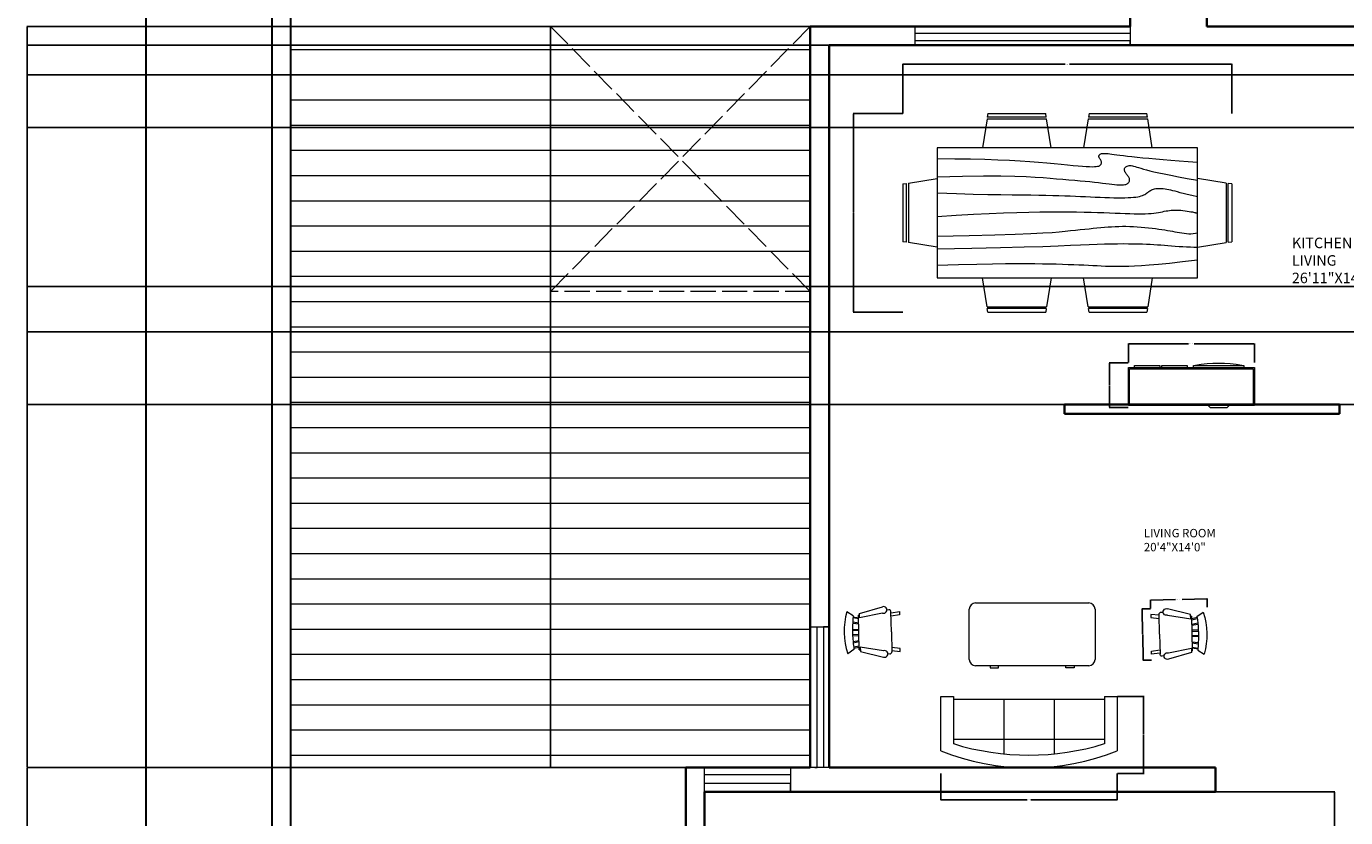
# Model space of a CAD drawing. Units: inches. Extents: x 727 to 1967, y -579 to 606.
# Tile 2 of 5: x 727 to 1355, y -78 to 299. Entities that reach past the tile are written whole.
import ezdxf

# ---------------------------------------------------------------- set-up
doc = ezdxf.new("R2010")
doc.units = ezdxf.units.IN
doc.header["$MEASUREMENT"] = 0
doc.linetypes.add('ACAD_ISO02W100', pattern=[15, 12, -3])
for name, color, linetype, lineweight in [('A-ANNO-DIMS', 2, 'Continuous', 18), ('A-AREA-IDEN', 7, 'Continuous', 18), ('A-FLOR-EXT', 7, 'Continuous', 25), ('A-FLOR-EXT-OVHD', 8, 'ACAD_ISO02W100', 18), ('A-FLOR-PATT', 9, 'Continuous', 13), ('A-FURN', 8, 'Continuous', 18), ('A-GLAZ', 4, 'Continuous', 18), ('A-WALL', 7, 'Continuous', 35), ('C-PROP', 7, 'Continuous', 30)]:
    doc.layers.add(name, color=color, linetype=linetype, lineweight=lineweight)
doc.styles.get("Standard").update_dxf_attribs({"font": 'arial.ttf'})
doc.dimstyles.get("Standard").update_dxf_attribs({"dimtxt": 0.18, "dimasz": 0.18, "dimexe": 0.18, "dimexo": 0.0625, "dimgap": 0.09, "dimtad": 0, "dimtih": 1, "dimtoh": 1, "dimdec": 4, "dimzin": 0, "dimdsep": 46, "dimtxsty": 'Standard', "dimcen": 0.09, "dimadec": 0, "dimazin": 0, "dimtfac": 1, "dimtdec": 4, "dimtofl": 0, "dimtmove": 0, "dimatfit": 3, "dimfxl": 1, "dimtolj": 1, "dimtzin": 0, "dimarcsym": 0})

# ---------------------------------------------------------------- blocks, each defined once
blk = doc.blocks.new('Dining Set - 36 x 72 in.')
for p, q in [((-22.2343, 26.00059), (-23.4847, 17.99762)), ((-22.2304, 26), (-5.7608, 26)), ((-22, 27.5), (-22.1562, 26.50042)), ((-5.8416, 26.5), (-22.1534, 26.5)), ((-22, 27.5), (-6, 27.5)), ((-5.8437, 26.49966), (-6, 27.5)), ((-4.5152, 17.99762), (-5.7655, 25.99926)), ((5.7657, 26.00059), (4.5153, 17.99762)), ((5.7696, 26), (22.2392, 26)), ((6, 27.5), (5.8438, 26.50042)), ((22.1584, 26.5), (5.8466, 26.5)), ((6, 27.5), (22, 27.5)), ((22.1563, 26.49966), (22, 27.5)), ((23.4848, 17.99762), (22.2345, 25.99926)), ((36, 18), (-36, 18)), ((-36, 18), (-36, -18)), ((36, -18), (36, 18)), ((-45.5, 8), (-44.5004, 8.15617)), ((-45.5, 8), (-45.5, -8)), ((-44.5, -8.15843), (-44.5, 8.15338)), ((-44.0006, 8.23428), (-35.9976, 9.48474)), ((-44, 8.23041), (-44, -8.23915)), ((44.0006, 8.23428), (35.9976, 9.48474)), ((44, 8.23041), (44, -8.23915)), ((44.5, -8.15843), (44.5, 8.15338)), ((45.5, 8), (44.5005, 8.15617)), ((45.5, 8), (45.5, -8)), ((-44.4997, -8.15631), (-45.5, -8)), ((-35.9976, -9.48476), (-43.9993, -8.2345)), ((35.9976, -9.48476), (43.9993, -8.2345)), ((44.4997, -8.15631), (45.5, -8)), ((-36, -18), (36, -18)), ((-22.2343, -26.0006), (-23.4847, -17.99762)), ((-4.5152, -17.99762), (-5.7655, -25.99928)), ((5.7657, -26.0006), (4.5153, -17.99762)), ((23.4848, -17.99762), (22.2345, -25.99928)), ((-22.2304, -26), (-5.7608, -26)), ((-22, -27.5), (-22.1562, -26.50044)), ((-5.8416, -26.5), (-22.1534, -26.5)), ((-22, -27.5), (-6, -27.5)), ((-5.8437, -26.49967), (-6, -27.5)), ((5.7696, -26), (22.2392, -26)), ((6, -27.5), (5.8438, -26.50044)), ((22.1584, -26.5), (5.8466, -26.5)), ((6, -27.5), (22, -27.5)), ((22.1563, -26.49967), (22, -27.5))]:
    blk.add_line(p, q)
for points in [[(-36, 15), (-31.1772, 14.97754), (-26.8079, 14.91406), (-22.8538, 14.81543), (-19.276, 14.6875), (-16.0362, 14.53613), (-13.0957, 14.36718), (-10.4159, 14.18652), (-7.9583, 14), (-5.6904, 13.81315), (-3.6035, 13.63021), (-1.6954, 13.45508), (0.0365, 13.29166), (1.5945, 13.14388), (2.9811, 13.01562), (4.1988, 12.9108), (5.25, 12.83333), (6.1393, 12.78613), (6.8802, 12.76823), (7.4883, 12.77767), (7.9792, 12.8125), (8.3685, 12.87077), (8.6719, 12.95052), (8.9049, 13.0498), (9.0833, 13.16666), (9.2205, 13.29899), (9.3216, 13.44401), (9.3895, 13.59879), (9.4271, 13.76041), (9.4373, 13.92594), (9.4232, 14.09245), (9.3875, 14.257), (9.3333, 14.41666), (9.2638, 14.56917), (9.1836, 14.71484), (9.0975, 14.85465), (9.0104, 14.98958), (8.9272, 15.1206), (8.8529, 15.2487), (8.7922, 15.37483), (8.75, 15.5), (8.7305, 15.62467), (8.7344, 15.74739), (8.7617, 15.86621), (8.8125, 15.97916), (8.8867, 16.08431), (8.9844, 16.17968), (9.1055, 16.26334), (9.25, 16.33333), (9.4189, 16.38802), (9.6172, 16.42708), (9.8506, 16.45052), (10.125, 16.45833), (10.4463, 16.45052), (10.8203, 16.42708), (11.2529, 16.38802), (11.75, 16.33333), (12.3184, 16.26318), (12.9694, 16.17838), (13.7151, 16.07991), (14.5677, 15.96875), (15.5395, 15.84586), (16.6426, 15.71224), (17.8893, 15.56884), (19.2917, 15.41666), (20.859, 15.25667), (22.5879, 15.08984), (24.4721, 14.91715), (26.5052, 14.73958), (28.6809, 14.5581), (30.9929, 14.3737), (33.4347, 14.18733), (36, 14)], [(-36, 10), (-28.9766, 10.14274), (-23.1725, 10.20442), (-18.4241, 10.19775), (-14.5677, 10.13541), (-11.4399, 10.03011), (-8.877, 9.89453), (-6.7154, 9.74137), (-4.7917, 9.58333), (-2.9698, 9.43082), (-1.2246, 9.28515), (0.4415, 9.14534), (2.026, 9.01041), (3.5266, 8.87939), (4.9408, 8.7513), (6.266, 8.62516), (7.5, 8.5), (8.6411, 8.37549), (9.6914, 8.2539), (10.6538, 8.13818), (11.5312, 8.03125), (12.3267, 7.93603), (13.043, 7.85547), (13.6831, 7.79248), (14.25, 7.75), (14.7471, 7.7303), (15.1797, 7.73307), (15.5537, 7.75732), (15.875, 7.80208), (16.1494, 7.86637), (16.3828, 7.94922), (16.5811, 8.04964), (16.75, 8.16666), (16.8944, 8.29915), (17.0143, 8.44531), (17.1089, 8.60319), (17.1771, 8.77083), (17.218, 8.94629), (17.2305, 9.1276), (17.2137, 9.31282), (17.1667, 9.5), (17.0895, 9.6875), (16.987, 9.875), (16.8649, 10.0625), (16.7292, 10.25), (16.5856, 10.4375), (16.4401, 10.625), (16.2985, 10.8125), (16.1667, 11), (16.05, 11.18733), (15.9518, 11.3737), (15.8752, 11.5581), (15.8229, 11.73958), (15.798, 11.91715), (15.8034, 12.08984), (15.842, 12.25667), (15.9167, 12.41666), (16.0295, 12.56836), (16.1784, 12.70833), (16.3605, 12.83268), (16.5729, 12.9375), (16.8127, 13.01888), (17.0768, 13.07291), (17.3625, 13.0957), (17.6667, 13.08333), (17.9894, 13.03312), (18.3418, 12.94726), (18.7382, 12.82918), (19.1927, 12.68229), (19.7195, 12.51001), (20.3327, 12.31575), (21.0465, 12.10294), (21.875, 11.875), (22.8357, 11.63354), (23.959, 11.37304), (25.2786, 11.08618), (26.8282, 10.76562), (28.6414, 10.40405), (30.752, 9.99414), (33.1936, 9.52856), (36, 9)], [(-36, 5.5), (-30.7157, 5.3348), (-26.069, 5.20963), (-21.9946, 5.11767), (-18.4271, 5.05208), (-15.3009, 5.00602), (-12.5508, 4.97265), (-10.1112, 4.94515), (-7.9167, 4.91666), (-5.909, 4.88167), (-4.0586, 4.83984), (-2.3429, 4.79215), (-0.7396, 4.73958), (0.7739, 4.6831), (2.22, 4.6237), (3.6213, 4.56233), (5, 4.5), (6.373, 4.43782), (7.7344, 4.3776), (9.0723, 4.32129), (10.375, 4.27083), (11.6309, 4.22819), (12.8281, 4.19531), (13.9551, 4.17415), (15, 4.16666), (15.954, 4.17448), (16.819, 4.19791), (17.6001, 4.23698), (18.3021, 4.29166), (18.9299, 4.36198), (19.4883, 4.44791), (19.9823, 4.54948), (20.4167, 4.66666), (20.7969, 4.79899), (21.1302, 4.94401), (21.4245, 5.09879), (21.6875, 5.26041), (21.9271, 5.42594), (22.1511, 5.59245), (22.3672, 5.757), (22.5834, 5.91666), (22.8065, 6.06868), (23.0404, 6.21093), (23.2879, 6.34147), (23.5521, 6.45833), (23.8358, 6.55957), (24.142, 6.64323), (24.4735, 6.70735), (24.8334, 6.75), (25.2235, 6.76969), (25.642, 6.76692), (26.0858, 6.74267), (26.5521, 6.69791), (27.0379, 6.63362), (27.5404, 6.55078), (28.0565, 6.45036), (28.5834, 6.33333), (29.1242, 6.19987), (29.7071, 6.04687), (30.3661, 5.87044), (31.1354, 5.66666), (32.0493, 5.43164), (33.142, 5.16146), (34.4475, 4.85221), (36, 4.5)], [(-36, -1), (-30.7915, -0.6591), (-26.0195, -0.38216), (-21.6519, -0.16284), (-17.6563, 0.00521), (-14.0005, 0.12833), (-10.6523, 0.21289), (-7.5796, 0.26522), (-4.75, 0.29166), (-2.134, 0.29793), (0.2878, 0.28711), (2.5317, 0.26163), (4.6146, 0.22396), (6.5529, 0.17651), (8.3633, 0.12174), (10.0623, 0.06209), (11.6667, 0), (13.1899, -0.06201), (14.6341, -0.1211), (15.9982, -0.17432), (17.2813, -0.21875), (18.4823, -0.25147), (19.6003, -0.26953), (20.6343, -0.27002), (21.5834, -0.25), (22.4481, -0.20768), (23.2357, -0.14584), (23.9549, -0.06836), (24.6146, 0.02083), (25.2235, 0.11784), (25.7904, 0.21875), (26.3241, 0.31966), (26.8334, 0.41666), (27.3265, 0.50618), (27.8099, 0.58593), (28.2894, 0.65397), (28.7709, 0.70833), (29.2601, 0.74707), (29.763, 0.76823), (30.2855, 0.76985), (30.8334, 0.75), (31.4088, 0.70784), (31.9994, 0.64713), (32.589, 0.57275), (33.1615, 0.48958), (33.7008, 0.4025), (34.1908, 0.3164), (34.6153, 0.23616), (34.9584, 0.16666), (35.2099, 0.11165), (35.3848, 0.07031), (35.504, 0.04069), (35.5886, 0.02083), (35.6594, 0.00879), (35.7377, 0.0026), (35.8442, 0.00032), (36, 0)], [(-36, -6.5), (-27.1843, -6.31267), (-20.084, -6.1263), (-14.469, -5.9419), (-10.1094, -5.76042), (-6.7752, -5.58285), (-4.2363, -5.41016), (-2.2629, -5.24333), (-0.625, -5.08334), (0.8708, -4.93099), (2.2715, -4.78646), (3.5872, -4.64974), (4.8281, -4.52084), (6.0046, -4.39974), (7.127, -4.28646), (8.2053, -4.18099), (9.25, -4.08334), (10.2705, -3.99382), (11.2734, -3.91407), (12.2647, -3.84603), (13.25, -3.79167), (14.2354, -3.75293), (15.2266, -3.73177), (16.2295, -3.73015), (17.25, -3.75), (18.2912, -3.79248), (19.3451, -3.85547), (20.4009, -3.93604), (21.4479, -4.03125), (22.4754, -4.13819), (23.4727, -4.25391), (24.4289, -4.37549), (25.3334, -4.5), (26.1785, -4.62492), (26.9694, -4.74935), (27.7145, -4.87281), (28.4219, -4.99479), (29.1, -5.11483), (29.7572, -5.23242), (30.4016, -5.34709), (31.0417, -5.45834), (31.6837, -5.56437), (32.3262, -5.65821), (32.9658, -5.73153), (33.599, -5.77604), (34.2224, -5.78345), (34.8327, -5.74545), (35.4264, -5.65373), (36, -5.5)], [(-36, -10), (-26.4022, -9.81299), (-18.4675, -9.62891), (-11.9839, -9.45069), (-6.7396, -9.28125), (-2.5226, -9.12354), (0.8789, -8.98047), (3.6769, -8.85498), (6.0833, -8.75), (8.2767, -8.66765), (10.3021, -8.60677), (12.1712, -8.56543), (13.8958, -8.54167), (15.4876, -8.53353), (16.9583, -8.53907), (18.3197, -8.55632), (19.5834, -8.58334), (20.7616, -8.61841), (21.8685, -8.66081), (22.9188, -8.71004), (23.9271, -8.76563), (24.9081, -8.82707), (25.8763, -8.89388), (26.8465, -8.96558), (27.8334, -9.04167), (28.8474, -9.12118), (29.8828, -9.20117), (30.93, -9.27824), (31.9792, -9.34896), (33.0205, -9.40991), (34.0443, -9.45768), (35.0407, -9.48885), (36, -9.5)], [(-36, -14.5), (-30.0881, -14.33513), (-25.0332, -14.21224), (-20.7312, -14.12647), (-17.0781, -14.07292), (-13.97, -14.04671), (-11.3027, -14.04297), (-8.9724, -14.05681), (-6.875, -14.08334), (-4.9224, -14.11833), (-3.0905, -14.16016), (-1.3709, -14.20785), (0.2448, -14.26042), (1.7647, -14.3169), (3.1973, -14.3763), (4.5507, -14.43767), (5.8333, -14.5), (7.0554, -14.5621), (8.235, -14.62175), (9.3922, -14.67652), (10.5469, -14.72396), (11.7192, -14.76164), (12.929, -14.78711), (14.1965, -14.79794), (15.5417, -14.79167), (16.9933, -14.76424), (18.6152, -14.70508), (20.4804, -14.60197), (22.6615, -14.44271), (25.2312, -14.21509), (28.2624, -13.9069), (31.8277, -13.50594), (36, -13)]]:
    blk.add_lwpolyline(points)
blk = doc.blocks.new('Entertainment Center')
for p, q in [((-4, 0), (-5, -1)), ((4, 0), (-4, 0)), ((5, -1), (4, 0)), ((-17, -19), (-17, -1)), ((-17, -1), (43, -1)), ((-16.5, -18.5), (-16.5, -1.5)), ((-16.5, -1.5), (42.5, -1.5)), ((42.5, -1.5), (42.5, -18.5)), ((43, -1), (43, -19)), ((42.5, -18.5), (-16.5, -18.5)), ((43, -19), (-17, -19)), ((-12, -20), (-12, -19)), ((12, -20), (-12, -20)), ((12, -19), (12, -20)), ((15, -20), (15, -19)), ((27, -20), (15, -20)), ((27, -19), (27, -20)), ((28, -20), (28, -19)), ((40, -20), (28, -20)), ((40, -19), (40, -20))]:
    blk.add_line(p, q)
blk.add_arc((0, 40), 61, 259.6111, 280.3889)
blk = doc.blocks.new('Sofa - Roundback 7 ft.')
for p, q in [((-36.000027, -34), (-36.000027, -11.4696)), ((-12.00002, -32.4421), (-12.00003, -6.5971)), ((11.99997, -32.4421), (11.99998, -6.5971)), ((35.99998, -34), (35.99998, -11.4696)), ((-35.999844, -13.3819), (35.9998, -13.3819)), ((-36.000027, -32.4421), (35.99998, -32.4421))]:
    blk.add_line(p, q)
for points in [[(-36.000027, -34), (-42.000027, -34), (-42.000027, -8)], [(41.99998, -8), (41.99998, -34), (35.99998, -34)]]:
    blk.add_lwpolyline(points)
for centre, radius, start, end in [((0, -114.25), 114.25, 68.43141, 111.5686), ((-0.00001, -127.1968), 121.1968, 72.72033, 107.2797)]:
    blk.add_arc(centre, radius, start, end)
blk = doc.blocks.new('Desk - 30 x 60 in.')
for p, q in [((-26.999995, 0), (26.999995, 0)), ((-29.999995, -27), (-29.999995, -3)), ((29.999995, -3), (29.999995, -27)), ((26.999995, -30), (-26.999995, -30)), ((-20.000005, -30), (-20.000005, -31)), ((-20.000005, -31), (-16.000005, -31)), ((-16.000005, -31), (-16.000005, -30)), ((15.999995, -31), (15.999995, -30)), ((19.999995, -31), (15.999995, -31)), ((19.999995, -30), (19.999995, -31))]:
    blk.add_line(p, q)
for centre, start, end in [((-26.499995, -3.5), 98.1301, 171.8699), ((26.499995, -3.5), 8.130102, 81.8699), ((-26.499995, -26.5), 188.1301, 261.8699), ((26.499995, -26.5), 278.1301, 351.8699)]:
    blk.add_arc(centre, 3.535534, start, end)
blk = doc.blocks.new('Chair - Rocking')
for p, q in [((-8, -4.5), (-10, -1.5)), ((-7.5, -4.5), (-7, -7)), ((-6.5, -7), (-7.02225, -4.43)), ((-4.5, -7), (-4.96674, -4.19951)), ((-4, -7), (-4.40532, -4.16272)), ((-1.5, -4.05012), (-1.5, -7)), ((-1, -7), (-1, -4.05012)), ((1, -7), (1, -4.04655)), ((1.5, -4.05012), (1.5, -7)), ((4, -7), (4.40187, -4.18694)), ((4.5, -7), (4.96761, -4.19437)), ((6.5, -7), (7, -4.4057)), ((7.5, -4.5), (7, -7)), ((8, -4.5), (10, -1.5)), ((-9, -7.5), (-12, -18.49999)), ((-7, -7.5), (-9, -7.5)), ((-9, -18.49999), (-7, -7.5)), ((-8.23428, -6.99939), (-8.3093, -7.47958)), ((-8.23041, -7), (8.23915, -7)), ((7, -7.5), (9, -7.5)), ((9, -18.49999), (7, -7.5)), ((8.31071, -7.48854), (8.23449, -7.00073)), ((9, -7.5), (12, -18.49999)), ((-10.36644, -20.64523), (-10.5, -21.49999)), ((-9, -22.49999), (-9.5, -26.49999)), ((0, -22.49999), (-9.5, -22.49999)), ((-8, -26.49999), (-7.5, -22.49999)), ((0, -22.49999), (9.5, -22.49999)), ((8, -26.49999), (7.5, -22.49999)), ((9, -22.49999), (9.5, -26.49999)), ((10.5, -21.49999), (10.3575, -20.58798)), ((-9.5, -26.49999), (-8, -26.49999)), ((9.5, -26.49999), (8, -26.49999))]:
    blk.add_line(p, q)
for centre, radius, start, end in [((0, -34.08333), 34.08333, 72.93847, 107.0615), ((0, -68.25004), 64.25, 93.92211, 97.15267), ((0, -68.25004), 64.25, 82.84733, 93.92211), ((-10.5, -18.99999), 1.58114, 161.5651, 18.43495), ((10.5, -18.99999), 1.58114, 161.5651, 18.43495), ((-9.5, -21.49999), 1, 180, 270), ((9.5, -21.49999), 1, 270, 0)]:
    blk.add_arc(centre, radius, start, end)
blk = doc.blocks.new('*D18')
at = {"layer": 'A-ANNO-DIMS', "color": 0, "lineweight": -2, "transparency": 16777216}
for p, q in [((1261.89, 21.78), (1261.8, 25.94)), ((1261.98, 25.77), (1273.73, 26.02)), ((1288.61, 26.35), (1276.87, 26.09)), ((1288.88, 22.37), (1288.79, 26.53))]:
    blk.add_line(p, q, dxfattribs=at)
at = {"layer": 'A-ANNO-DIMS', "color": 0, "transparency": 16777216}
for points in [[(1261.98, 25.8), (1261.98, 25.74), (1261.8, 25.76)], [(1288.61, 26.38), (1288.61, 26.32), (1288.79, 26.35)]]:
    blk.add_solid(points, dxfattribs=at)
at = {"layer": 'Defpoints', "color": 0, "transparency": 16777216}
for p in [(1288.79, 26.35), (1261.89, 21.71), (1288.88, 22.3)]:
    blk.add_point(p, dxfattribs=at)
at = {"layer": 'A-ANNO-DIMS', "color": 0, "transparency": 16777216, "insert": (1275.3, 26.06), "char_height": 0.18, "attachment_point": 5}
blk.add_mtext('\\A1;ROCKING CHAIR 27 TYP.', dxfattribs=at)
blk = doc.blocks.new('*D19')
at = {"layer": 'A-ANNO-DIMS', "color": 0, "lineweight": -2, "transparency": 16777216}
for p, q in [((1261.83, 21.71), (1257.66, 21.62)), ((1257.84, 21.45), (1258.1, 9.59)), ((1258.37, -2.62), (1258.11, 9.23)), ((1262.36, -2.72), (1258.19, -2.81))]:
    blk.add_line(p, q, dxfattribs=at)
at = {"layer": 'A-ANNO-DIMS', "color": 0, "transparency": 16777216}
for points in [[(1257.87, 21.45), (1257.81, 21.45), (1257.84, 21.63)], [(1258.4, -2.62), (1258.34, -2.62), (1258.37, -2.8)]]:
    blk.add_solid(points, dxfattribs=at)
at = {"layer": 'Defpoints', "color": 0, "transparency": 16777216}
for p in [(1257.84, 21.63), (1261.89, 21.71), (1262.42, -2.71)]:
    blk.add_point(p, dxfattribs=at)
at = {"layer": 'A-ANNO-DIMS', "color": 0, "transparency": 16777216, "insert": (1258.11, 9.41), "char_height": 0.18, "attachment_point": 5}
blk.add_mtext('\\A1;24 TYP.', dxfattribs=at)
blk = doc.blocks.new('*D22')
at = {"layer": 'A-ANNO-DIMS', "color": 0, "lineweight": -2, "transparency": 16777216}
for p, q in [((1161.98, -56.76), (1161.98, -69.47)), ((1245.98, -56.76), (1245.98, -69.47)), ((1162.16, -69.29), (1203.08, -69.29)), ((1245.8, -69.29), (1204.89, -69.29))]:
    blk.add_line(p, q, dxfattribs=at)
at = {"layer": 'A-ANNO-DIMS', "color": 0, "transparency": 16777216}
for points in [[(1162.16, -69.26), (1162.16, -69.32), (1161.98, -69.29)], [(1245.8, -69.26), (1245.8, -69.32), (1245.98, -69.29)]]:
    blk.add_solid(points, dxfattribs=at)
at = {"layer": 'Defpoints', "color": 0, "transparency": 16777216}
for p in [(1161.98, -56.69), (1245.98, -56.69), (1161.98, -69.29)]:
    blk.add_point(p, dxfattribs=at)
at = {"layer": 'A-ANNO-DIMS', "color": 0, "transparency": 16777216, "insert": (1203.98, -69.29), "char_height": 0.18, "attachment_point": 5}
blk.add_mtext('\\A1;SOFA 84 TYP.', dxfattribs=at)
blk = doc.blocks.new('*D23')
at = {"layer": 'A-ANNO-DIMS', "color": 0, "lineweight": -2, "transparency": 16777216}
for p, q in [((1246.05, -20.03), (1258.76, -20.03)), ((1258.58, -20.21), (1258.58, -38.18)), ((1258.58, -56.51), (1258.58, -38.54)), ((1246.05, -56.69), (1258.76, -56.69))]:
    blk.add_line(p, q, dxfattribs=at)
at = {"layer": 'A-ANNO-DIMS', "color": 0, "transparency": 16777216}
for points in [[(1258.55, -20.21), (1258.61, -20.21), (1258.58, -20.03)], [(1258.55, -56.51), (1258.61, -56.51), (1258.58, -56.69)]]:
    blk.add_solid(points, dxfattribs=at)
at = {"layer": 'Defpoints', "color": 0, "transparency": 16777216}
for p in [(1245.98, -20.03), (1245.98, -56.69), (1258.58, -56.69)]:
    blk.add_point(p, dxfattribs=at)
at = {"layer": 'A-ANNO-DIMS', "color": 0, "transparency": 16777216, "insert": (1258.58, -38.36), "char_height": 0.18, "attachment_point": 5}
blk.add_mtext('\\A1;37 TYP.', dxfattribs=at)
blk = doc.blocks.new('*D24')
at = {"layer": 'A-ANNO-DIMS', "color": 0, "lineweight": -2, "transparency": 16777216}
for p, q in [((1251.29, 138.91), (1251.29, 148.03)), ((1251.47, 147.85), (1280.01, 147.85)), ((1311.11, 147.85), (1282.58, 147.85)), ((1311.29, 138.91), (1311.29, 148.03))]:
    blk.add_line(p, q, dxfattribs=at)
at = {"layer": 'A-ANNO-DIMS', "color": 0, "transparency": 16777216}
for points in [[(1251.47, 147.88), (1251.47, 147.82), (1251.29, 147.85)], [(1311.11, 147.88), (1311.11, 147.82), (1311.29, 147.85)]]:
    blk.add_solid(points, dxfattribs=at)
at = {"layer": 'Defpoints', "color": 0, "transparency": 16777216}
for p in [(1251.29, 147.85), (1251.29, 138.85), (1311.29, 138.85)]:
    blk.add_point(p, dxfattribs=at)
at = {"layer": 'A-ANNO-DIMS', "color": 0, "transparency": 16777216, "insert": (1281.29, 147.85), "char_height": 0.18, "attachment_point": 5}
blk.add_mtext('\\A1;MEDIA UNIT 60 TYP.', dxfattribs=at)
blk = doc.blocks.new('*D25')
at = {"layer": 'A-ANNO-DIMS', "color": 0, "lineweight": -2, "transparency": 16777216}
for p, q in [((1251.23, 138.85), (1242.11, 138.85)), ((1242.29, 138.67), (1242.29, 128.36)), ((1242.29, 117.7), (1242.29, 128)), ((1251.23, 117.52), (1242.11, 117.52))]:
    blk.add_line(p, q, dxfattribs=at)
at = {"layer": 'A-ANNO-DIMS', "color": 0, "transparency": 16777216}
for points in [[(1242.26, 138.67), (1242.32, 138.67), (1242.29, 138.85)], [(1242.26, 117.7), (1242.32, 117.7), (1242.29, 117.52)]]:
    blk.add_solid(points, dxfattribs=at)
at = {"layer": 'Defpoints', "color": 0, "transparency": 16777216}
for p in [(1251.29, 138.85), (1242.29, 117.52), (1251.29, 117.52)]:
    blk.add_point(p, dxfattribs=at)
at = {"layer": 'A-ANNO-DIMS', "color": 0, "transparency": 16777216, "insert": (1242.29, 128.18), "char_height": 0.18, "attachment_point": 5}
blk.add_mtext('\\A1;21 TYP.', dxfattribs=at)
blk = doc.blocks.new('*D34')
at = {"layer": 'A-ANNO-DIMS', "color": 0, "lineweight": -2, "transparency": 16777216}
for p, q in [((1143.97, 257.6), (1143.97, 281.2)), ((1144.15, 281.02), (1221.21, 281.02)), ((1300.34, 281.02), (1223.28, 281.02)), ((1300.52, 257.6), (1300.52, 281.2))]:
    blk.add_line(p, q, dxfattribs=at)
at = {"layer": 'A-ANNO-DIMS', "color": 0, "transparency": 16777216}
for points in [[(1144.15, 281.05), (1144.15, 280.99), (1143.97, 281.02)], [(1300.34, 281.05), (1300.34, 280.99), (1300.52, 281.02)]]:
    blk.add_solid(points, dxfattribs=at)
at = {"layer": 'Defpoints', "color": 0, "transparency": 16777216}
for p in [(1300.52, 281.02), (1143.97, 257.54), (1300.52, 257.54)]:
    blk.add_point(p, dxfattribs=at)
at = {"layer": 'A-ANNO-DIMS', "color": 0, "transparency": 16777216, "insert": (1222.25, 281.02), "char_height": 0.18, "attachment_point": 5}
blk.add_mtext('\\A1;DINING SET 157', dxfattribs=at)
blk = doc.blocks.new('*D35')
at = {"layer": 'A-ANNO-DIMS', "color": 0, "lineweight": -2, "transparency": 16777216}
for p, q in [((1143.91, 257.54), (1120.31, 257.54)), ((1120.49, 257.36), (1120.49, 210.41)), ((1120.49, 163.1), (1120.49, 210.05)), ((1143.91, 162.92), (1120.31, 162.92))]:
    blk.add_line(p, q, dxfattribs=at)
at = {"layer": 'A-ANNO-DIMS', "color": 0, "transparency": 16777216}
for points in [[(1120.46, 257.36), (1120.52, 257.36), (1120.49, 257.54)], [(1120.46, 163.1), (1120.52, 163.1), (1120.49, 162.92)]]:
    blk.add_solid(points, dxfattribs=at)
at = {"layer": 'Defpoints', "color": 0, "transparency": 16777216}
for p in [(1120.49, 257.54), (1143.97, 257.54), (1143.97, 162.92)]:
    blk.add_point(p, dxfattribs=at)
at = {"layer": 'A-ANNO-DIMS', "color": 0, "transparency": 16777216, "insert": (1120.49, 210.23), "char_height": 0.18, "attachment_point": 5}
blk.add_mtext('\\A1;95', dxfattribs=at)
blk = doc.blocks.new('*D47')
at = {"layer": 'A-ANNO-DIMS', "color": 0, "lineweight": -2, "transparency": 16777216}
for p, q in [((852.52, 299.02), (726.8, 299.02)), ((726.98, 298.84), (726.98, 122.7)), ((726.98, -53.8), (726.98, 122.33)), ((852.52, -53.98), (726.8, -53.98))]:
    blk.add_line(p, q, dxfattribs=at)
at = {"layer": 'A-ANNO-DIMS', "color": 0, "transparency": 16777216}
for points in [[(726.95, 298.84), (727.01, 298.84), (726.98, 299.02)], [(726.95, -53.8), (727.01, -53.8), (726.98, -53.98)]]:
    blk.add_solid(points, dxfattribs=at)
at = {"layer": 'Defpoints', "color": 0, "transparency": 16777216}
for p in [(852.58, 299.02), (726.98, -53.98), (852.58, -53.98)]:
    blk.add_point(p, dxfattribs=at)
at = {"layer": 'A-ANNO-DIMS', "color": 0, "transparency": 16777216, "insert": (726.98, 122.52), "char_height": 0.18, "attachment_point": 5}
blk.add_mtext('\\A1;353', dxfattribs=at)
blk = doc.blocks.new('*D48')
at = {"layer": 'A-ANNO-DIMS', "color": 0, "lineweight": -2, "transparency": 16777216}
for p, q in [((852.52, -53.98), (726.8, -53.98)), ((726.98, -54.16), (726.98, -152.55)), ((726.98, -251.3), (726.98, -152.92)), ((950.28, -251.48), (726.8, -251.48))]:
    blk.add_line(p, q, dxfattribs=at)
at = {"layer": 'A-ANNO-DIMS', "color": 0, "transparency": 16777216}
for points in [[(726.95, -54.16), (727.01, -54.16), (726.98, -53.98)], [(726.95, -251.3), (727.01, -251.3), (726.98, -251.48)]]:
    blk.add_solid(points, dxfattribs=at)
at = {"layer": 'Defpoints', "color": 0, "transparency": 16777216}
for p in [(852.58, -53.98), (726.98, -251.48), (950.34, -251.48)]:
    blk.add_point(p, dxfattribs=at)
at = {"layer": 'A-ANNO-DIMS', "color": 0, "transparency": 16777216, "insert": (726.98, -152.73), "char_height": 0.18, "attachment_point": 5}
blk.add_mtext('\\A1;197.5', dxfattribs=at)
blk = doc.blocks.new('*D59')
at = {"layer": 'A-ANNO-DIMS', "color": 0, "lineweight": -2, "transparency": 16777216}
for p, q in [((1292.91, -65.48), (1349.63, -65.48)), ((1349.45, -65.66), (1349.45, -95.86)), ((1349.45, -126.41), (1349.45, -96.22)), ((1292.91, -126.59), (1349.63, -126.59))]:
    blk.add_line(p, q, dxfattribs=at)
at = {"layer": 'A-ANNO-DIMS', "color": 0, "transparency": 16777216}
for points in [[(1349.42, -65.66), (1349.48, -65.66), (1349.45, -65.48)], [(1349.42, -126.41), (1349.48, -126.41), (1349.45, -126.59)]]:
    blk.add_solid(points, dxfattribs=at)
at = {"layer": 'Defpoints', "color": 0, "transparency": 16777216}
for p in [(1292.85, -65.48), (1292.85, -126.59), (1349.45, -126.59)]:
    blk.add_point(p, dxfattribs=at)
at = {"layer": 'A-ANNO-DIMS', "color": 0, "transparency": 16777216, "insert": (1349.45, -96.04), "char_height": 0.18, "attachment_point": 5}
blk.add_mtext('\\A1;61.1', dxfattribs=at)
blk = doc.blocks.new('*D69')
at = {"layer": 'A-ANNO-DIMS', "color": 0, "lineweight": -2, "transparency": 16777216}
for p, q in [((1615.78, 290.02), (726.8, 290.02)), ((726.98, 289.84), (726.98, 283.18)), ((726.98, 276.17), (726.98, 282.82)), ((1615.78, 275.99), (726.8, 275.99))]:
    blk.add_line(p, q, dxfattribs=at)
at = {"layer": 'A-ANNO-DIMS', "color": 0, "transparency": 16777216}
for points in [[(726.95, 289.84), (727.01, 289.84), (726.98, 290.02)], [(726.95, 276.17), (727.01, 276.17), (726.98, 275.99)]]:
    blk.add_solid(points, dxfattribs=at)
at = {"layer": 'Defpoints', "color": 0, "transparency": 16777216}
for p in [(1615.85, 290.02), (726.98, 275.99), (1615.85, 275.99)]:
    blk.add_point(p, dxfattribs=at)
at = {"layer": 'A-ANNO-DIMS', "color": 0, "transparency": 16777216, "insert": (726.98, 283), "char_height": 0.18, "attachment_point": 5}
blk.add_mtext('\\A1;14.027', dxfattribs=at)
blk = doc.blocks.new('*D70')
at = {"layer": 'A-ANNO-DIMS', "color": 0, "lineweight": -2, "transparency": 16777216}
for p, q in [((1615.78, 275.99), (726.8, 275.99)), ((726.98, 275.81), (726.98, 263.6)), ((726.98, 251.03), (726.98, 263.24)), ((1615.78, 250.85), (726.8, 250.85))]:
    blk.add_line(p, q, dxfattribs=at)
at = {"layer": 'A-ANNO-DIMS', "color": 0, "transparency": 16777216}
for points in [[(726.95, 275.81), (727.01, 275.81), (726.98, 275.99)], [(726.95, 251.03), (727.01, 251.03), (726.98, 250.85)]]:
    blk.add_solid(points, dxfattribs=at)
at = {"layer": 'Defpoints', "color": 0, "transparency": 16777216}
for p in [(1615.85, 275.99), (726.98, 250.85), (1615.85, 250.85)]:
    blk.add_point(p, dxfattribs=at)
at = {"layer": 'A-ANNO-DIMS', "color": 0, "transparency": 16777216, "insert": (726.98, 263.42), "char_height": 0.18, "attachment_point": 5}
blk.add_mtext('\\A1;25.135', dxfattribs=at)
blk = doc.blocks.new('*D71')
at = {"layer": 'A-ANNO-DIMS', "color": 0, "lineweight": -2, "transparency": 16777216}
for p, q in [((1615.78, 250.85), (726.8, 250.85)), ((726.98, 250.67), (726.98, 213.22)), ((726.98, 175.39), (726.98, 212.85)), ((1615.78, 175.21), (726.8, 175.21))]:
    blk.add_line(p, q, dxfattribs=at)
at = {"layer": 'A-ANNO-DIMS', "color": 0, "transparency": 16777216}
for points in [[(726.95, 250.67), (727.01, 250.67), (726.98, 250.85)], [(726.95, 175.39), (727.01, 175.39), (726.98, 175.21)]]:
    blk.add_solid(points, dxfattribs=at)
at = {"layer": 'Defpoints', "color": 0, "transparency": 16777216}
for p in [(1615.85, 250.85), (726.98, 175.21), (1615.85, 175.21)]:
    blk.add_point(p, dxfattribs=at)
at = {"layer": 'A-ANNO-DIMS', "color": 0, "transparency": 16777216, "insert": (726.98, 213.03), "char_height": 0.18, "attachment_point": 5}
blk.add_mtext('\\A1;75.64', dxfattribs=at)
blk = doc.blocks.new('*D72')
at = {"layer": 'A-ANNO-DIMS', "color": 0, "lineweight": -2, "transparency": 16777216}
for p, q in [((1615.78, 175.21), (726.8, 175.21)), ((726.98, 175.03), (726.98, 164.56)), ((726.98, 153.73), (726.98, 164.2)), ((1615.78, 153.55), (726.8, 153.55))]:
    blk.add_line(p, q, dxfattribs=at)
at = {"layer": 'A-ANNO-DIMS', "color": 0, "transparency": 16777216}
for points in [[(726.95, 175.03), (727.01, 175.03), (726.98, 175.21)], [(726.95, 153.73), (727.01, 153.73), (726.98, 153.55)]]:
    blk.add_solid(points, dxfattribs=at)
at = {"layer": 'Defpoints', "color": 0, "transparency": 16777216}
for p in [(1615.85, 175.21), (726.98, 153.55), (1615.85, 153.55)]:
    blk.add_point(p, dxfattribs=at)
at = {"layer": 'A-ANNO-DIMS', "color": 0, "transparency": 16777216, "insert": (726.98, 164.38), "char_height": 0.18, "attachment_point": 5}
blk.add_mtext('\\A1;21.67', dxfattribs=at)
blk = doc.blocks.new('*D73')
at = {"layer": 'A-ANNO-DIMS', "color": 0, "lineweight": -2, "transparency": 16777216}
for p, q in [((1615.78, 153.55), (726.8, 153.55)), ((726.98, 153.37), (726.98, 136.46)), ((726.98, 119.2), (726.98, 136.1)), ((1615.78, 119.02), (726.8, 119.02))]:
    blk.add_line(p, q, dxfattribs=at)
at = {"layer": 'A-ANNO-DIMS', "color": 0, "transparency": 16777216}
for points in [[(726.95, 153.37), (727.01, 153.37), (726.98, 153.55)], [(726.95, 119.2), (727.01, 119.2), (726.98, 119.02)]]:
    blk.add_solid(points, dxfattribs=at)
at = {"layer": 'Defpoints', "color": 0, "transparency": 16777216}
for p in [(1615.85, 153.55), (726.98, 119.02), (1615.85, 119.02)]:
    blk.add_point(p, dxfattribs=at)
at = {"layer": 'A-ANNO-DIMS', "color": 0, "transparency": 16777216, "insert": (726.98, 136.28), "char_height": 0.18, "attachment_point": 5}
blk.add_mtext('\\A1;34.53', dxfattribs=at)

msp = doc.modelspace()

# ---------------------------------------------------------------- hatches: boundary and pattern name
at = {"layer": 'A-FLOR-PATT'}
h = msp.add_hatch(dxfattribs=at)
h.set_pattern_fill('ANSI31', color=256, scale=96, angle=315, style=0)
h.paths.add_polyline_path([(1099.8463, -53.9849), (1099.8463, 299.0151), (852.5815, 299.0151), (852.5815, -53.9849)])

# ---------------------------------------------------------------- linework, layer by layer
at = {"layer": 'A-FLOR-EXT'}
for p, q in [((852.5815, 299.0151), (1099.8463, 299.0151)), ((976.2139, 299.0151), (976.2139, -53.9849)), ((1099.8463, -53.9849), (852.5815, -53.9849))]:
    msp.add_line(p, q, dxfattribs=at)
at = {"layer": 'A-FLOR-EXT-OVHD'}
for p, q in [((976.2139, 172.7192), (1099.8463, 299.0151)), ((1099.8463, 172.7192), (976.2139, 299.0151)), ((1099.8463, 172.7192), (976.2139, 172.7192))]:
    msp.add_line(p, q, dxfattribs=at)
at = {"layer": 'A-GLAZ'}
for p, q in [((1149.8197, 290.0151), (1149.8197, 299.0151)), ((1149.8197, 299.0151), (1252.1653, 299.0151)), ((1149.8197, 292.1597), (1149.8197, 295.732)), ((1149.8197, 295.732), (1252.1653, 295.732)), ((1252.1653, 299.0151), (1252.1653, 290.0151)), ((1252.1653, 292.1597), (1149.8197, 292.1597)), ((1252.1653, 290.0151), (1252.1653, 292.1597)), ((1099.8463, -53.9849), (1099.8463, 13.1355)), ((1099.8463, 13.1355), (1108.8463, 13.1355)), ((1103.1183, -53.9849), (1103.1183, 13.1355)), ((1107.1683, 13.1355), (1106.2082, 13.1355)), ((1106.2082, 13.1355), (1106.2082, -53.9849)), ((1108.8463, 13.1355), (1107.1683, 13.1355)), ((1049.5236, -65.4849), (1049.5236, -53.9849)), ((1049.5236, -53.9849), (1090.3627, -53.9849)), ((1090.3627, -53.9849), (1090.3627, -65.4849)), ((1108.8463, -53.9849), (1099.8463, -53.9849)), ((1106.2082, -53.9849), (1102.0789, -53.9849)), ((1102.0789, -53.9849), (1103.1183, -53.9849)), ((1049.5236, -61.574), (1049.5236, -57.2759)), ((1049.5236, -57.2759), (1090.3627, -57.2759)), ((1090.3627, -61.574), (1049.5236, -61.574)), ((1090.3627, -63.4059), (1090.3627, -61.574)), ((1090.3627, -65.4849), (1090.3627, -63.4059))]:
    msp.add_line(p, q, dxfattribs=at)
at = {"layer": 'A-WALL'}
for p, q in [((1252.1653, 299.0151), (1252.1653, 333.0244)), ((1288.6382, 333.0244), (1288.6382, 299.0151)), ((1099.8463, 299.0151), (1252.1653, 299.0151)), ((1099.8463, 299.0151), (1099.8463, -53.9849)), ((1252.1653, 299.0151), (1099.8463, 299.0151)), ((1735.3463, 299.0151), (1288.6382, 299.0151)), ((1288.6382, 299.0151), (1339.8463, 299.0151)), ((1283.8463, 290.0151), (1108.8463, 290.0151)), ((1108.8463, -53.9849), (1108.8463, 290.0151)), ((1615.8463, 290.0151), (1283.8463, 290.0151)), ((1345.2945, 290.0151), (1405.2835, 290.0151)), ((1220.9049, 114.5151), (1220.9049, 119.0151)), ((1220.9049, 119.0151), (1351.833, 119.0151)), ((1351.833, 119.0151), (1220.9049, 119.0151)), ((1351.833, 114.5151), (1220.9049, 114.5151)), ((1351.833, 119.0151), (1351.833, 114.5151)), ((1040.5236, -251.4849), (1040.5236, -53.9849)), ((1040.5236, -53.9849), (1099.8463, -53.9849)), ((1292.8463, -53.9849), (1108.8463, -53.9849)), ((1108.8463, -53.9849), (1119.0718, -53.9849)), ((1292.8463, -53.9849), (1292.8463, -65.4849)), ((1292.8463, -65.4849), (1049.5236, -65.4849)), ((1049.5236, -242.4849), (1049.5236, -65.4849))]:
    msp.add_line(p, q, dxfattribs=at)
at = {"layer": 'C-PROP'}
for p, q in [((783.5815, -461.8103), (783.5815, 392.0151)), ((843.5815, 299.0151), (843.5815, 392.0151)), ((852.5815, 299.0151), (852.5815, 359.0151)), ((843.5815, -521.8103), (843.5815, 299.0151)), ((852.5815, -512.8103), (852.5815, 299.0151))]:
    msp.add_line(p, q, dxfattribs=at)

# ---------------------------------------------------------------- block references
at = {"layer": 'A-FURN', "xscale": 1.720335708863012, "yscale": 1.720335708863012, "zscale": 1.720335708863012}
msp.add_blockref('Dining Set - 36 x 72 in.', (1222.2454, 210.2307), dxfattribs=at)
at = {"layer": 'A-FURN'}
for name, p, rotation in [('Entertainment Center', (1294.293, 117.5151), 180), ('Chair - Rocking', (1115.9874, 10.24), 91.2499944704987), ('Sofa - Roundback 7 ft.', (1203.9826, -54.0279), 180)]:
    msp.add_blockref(name, p, dxfattribs=dict(at, rotation=rotation))
msp.add_blockref('Desk - 30 x 60 in.', (1205.4937, 24.5195), dxfattribs=at)
at = {"layer": 'A-FURN', "xscale": -1, "rotation": 271.2499944704995}
msp.add_blockref('Chair - Rocking', (1288.6487, 10.0783), dxfattribs=at)

# ---------------------------------------------------------------- texts
at = {"layer": 'A-AREA-IDEN', "attachment_point": 1}
for s, insert, char_height in [('KITCHEN /\\PLIVING\\P26\'11"X14\'0"', (1329.1678, 198.3978), 5), ('LIVING ROOM\\P20\'4"X14\'0"', (1258.6645, 59.7085), 4)]:
    msp.add_mtext_dynamic_manual_height_columns(s, width=588.620786, gutter_width=1, heights=[0], dxfattribs=dict(at, insert=insert, char_height=char_height))

# ---------------------------------------------------------------- dimensions: what is measured, and where the dimension line sits
at = {"layer": 'A-ANNO-DIMS'}
for base, p1, p2, angle, override, picture, middle in [((726.9815, -53.9849), (852.5815, 299.0151), (852.5815, -53.9849), 90, {"dimdec": 0, "dimlfac": 1, "dimrnd": 0, "dimzin": 0, "dimdsep": 46, "dimlunit": 2}, '*D47', (726.9815, 122.5151)), ((726.9815, 275.988), (1615.8463, 290.0151), (1615.8463, 275.988), 90, {"dimdec": 3, "dimlfac": 1, "dimrnd": 0, "dimzin": 0, "dimdsep": 46, "dimlunit": 2}, '*D69', (726.9815, 283.0015)), ((726.9815, 250.8534), (1615.8463, 275.988), (1615.8463, 250.8534), 90, {"dimdec": 3, "dimlfac": 1, "dimrnd": 0, "dimzin": 0, "dimdsep": 46, "dimlunit": 2}, '*D70', (726.9815, 263.4207)), ((1120.4875, 257.54), (1143.9701, 162.9215), (1143.9701, 257.54), 90, {"dimdec": 0, "dimlfac": 1, "dimrnd": 0, "dimzin": 0, "dimdsep": 46, "dimlunit": 2}, '*D35', (1120.4875, 210.2307)), ((726.9815, 175.2149), (1615.8463, 250.8534), (1615.8463, 175.2149), 90, {"dimdec": 2, "dimlfac": 1, "dimrnd": 0, "dimzin": 0, "dimdsep": 46, "dimlunit": 2}, '*D71', (726.9815, 213.0341)), ((726.9815, 153.5464), (1615.8463, 175.2149), (1615.8463, 153.5464), 90, {"dimdec": 2, "dimlfac": 1, "dimrnd": 0, "dimzin": 0, "dimdsep": 46, "dimlunit": 2}, '*D72', (726.9815, 164.3806)), ((726.9815, 119.0151), (1615.8463, 153.5464), (1615.8463, 119.0151), 90, {"dimdec": 2, "dimlfac": 1, "dimrnd": 0, "dimzin": 0, "dimdsep": 46, "dimlunit": 2}, '*D73', (726.9815, 136.2808)), ((726.9815, -251.4849), (852.5815, -53.9849), (950.3408, -251.4849), 90, {"dimdec": 1, "dimlfac": 1, "dimrnd": 0, "dimzin": 0, "dimdsep": 46, "dimlunit": 2}, '*D48', (726.9815, -152.7349)), ((1349.4463, -126.5894), (1292.8463, -65.4849), (1292.8463, -126.5894), 270, {"dimdec": 1, "dimlfac": 1, "dimrnd": 0, "dimzin": 0, "dimdsep": 46, "dimlunit": 2}, '*D59', (1349.4463, -96.0371))]:
    dim = msp.add_linear_dim(base=base, p1=p1, p2=p2, angle=angle, dimstyle='Standard', override=override, dxfattribs=at)
    dim.commit()
    dim.dimension.update_dxf_attribs({"geometry": picture, "text_midpoint": middle})
dim = msp.add_linear_dim(base=(1300.5207, 281.0225), p1=(1143.9701, 257.54), p2=(1300.5207, 257.54), text='DINING SET <>', dimstyle='Standard', override={"dimdec": 0, "dimlfac": 1, "dimrnd": 0, "dimzin": 0, "dimdsep": 46, "dimlunit": 2}, dxfattribs=at)
dim.commit()
dim.dimension.update_dxf_attribs({"geometry": '*D34', "text_midpoint": (1222.2454, 281.0225)})
for base, p1, p2, angle, text, picture, middle in [((1251.293, 147.8485), (1311.293, 138.8485), (1251.293, 138.8485), 180, 'MEDIA UNIT <> TYP.', '*D24', (1281.293, 147.8485)), ((1242.293, 117.5151), (1251.293, 138.8485), (1251.293, 117.5151), 270, '<> TYP.', '*D25', (1242.293, 128.1818)), ((1288.7937, 26.3529), (1261.8885, 21.7148), (1288.882, 22.3038), 1.2499945, 'ROCKING CHAIR <> TYP.', '*D18', (1275.2969, 26.0584)), ((1257.8394, 21.6265), (1262.4215, -2.7145), (1261.8885, 21.7148), 91.2499945, '<> TYP.', '*D19', (1258.1059, 9.4118)), ((1258.5826, -56.6946), (1245.9826, -20.0279), (1245.9826, -56.6946), 270, '<> TYP.', '*D23', (1258.5826, -38.3613)), ((1161.9826, -69.2946), (1245.9826, -56.6946), (1161.9826, -56.6946), 180, 'SOFA <> TYP.', '*D22', (1203.9826, -69.2946))]:
    dim = msp.add_linear_dim(base=base, p1=p1, p2=p2, angle=angle, text=text, dimstyle='Standard', override={"dimdec": 0, "dimlfac": 1, "dimrnd": 0, "dimzin": 0, "dimdsep": 46, "dimlunit": 2}, dxfattribs=at)
    dim.commit()
    dim.dimension.update_dxf_attribs({"geometry": picture, "text_midpoint": middle})

doc.saveas('drawing.dxf')
